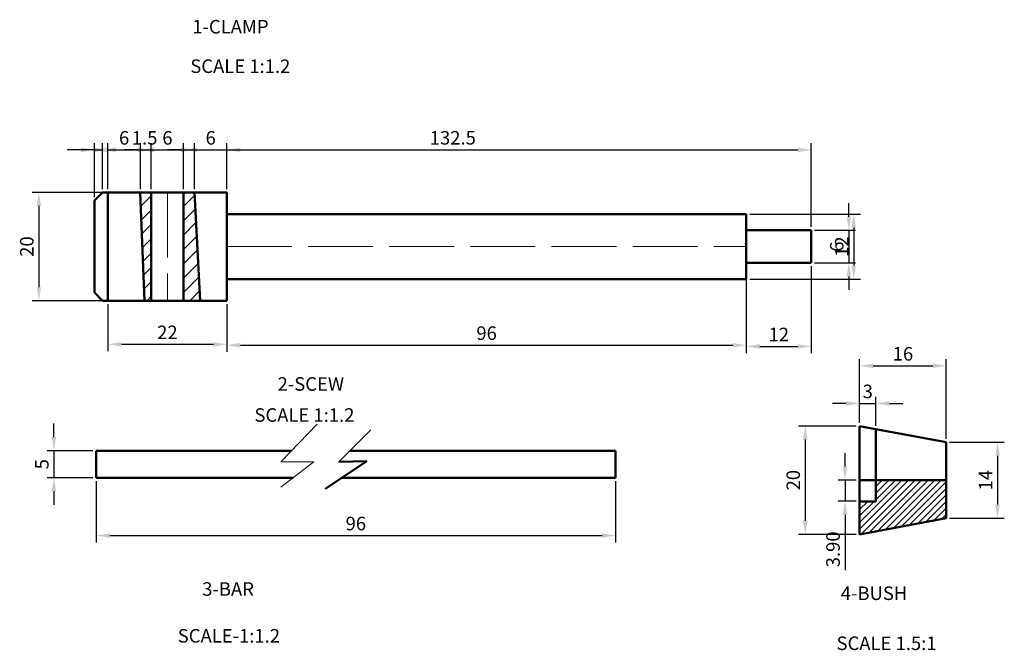
# Model space of a CAD drawing. Units: millimetres. Extents: x 1139 to 1488, y 1435 to 1756.
# Tile 1 of 3: x 1152 to 1334, y 1489 to 1606. Entities that reach past the tile are written whole.
import ezdxf

# ---------------------------------------------------------------- set-up
doc = ezdxf.new("R2010")
doc.units = ezdxf.units.MM
doc.linetypes.add('ACAD_ISO02W100', pattern=[15, 12, -3])
for name, color, linetype, lineweight in [('M-BREAK', 8, 'ACAD_ISO02W100', 18), ('M-CNTR', 4, 'ACAD_ISO02W100', 18), ('M-DIMS', 2, 'Continuous', 25), ('M-HATC', 8, 'Continuous', 18), ('M-OUTL', 7, 'Continuous', 50), ('M-TEXT', 7, 'Continuous', 25)]:
    doc.layers.add(name, color=color, linetype=linetype, lineweight=lineweight)
doc.styles.get("Standard").update_dxf_attribs({"font": 'arial.ttf'})
doc.dimstyles.new('ISO-25', dxfattribs={"dimtxt": 2.5, "dimasz": 2.5, "dimexe": 1.25, "dimexo": 0.625, "dimtad": 1, "dimtxsty": 'Standard', "dimcen": 2.5, "dimadec": 0, "dimazin": 0, "dimtfac": 1, "dimtmove": 0, "dimatfit": 3, "dimfxl": 1, "dimarcsym": 0})

# ---------------------------------------------------------------- blocks, each defined once
blk = doc.blocks.new('*D11')
at = {"layer": 'Defpoints', "color": 0, "transparency": 16777216}
for p in [(1168, 1554), (1190, 1554), (1190, 1545.95)]:
    blk.add_point(p, dxfattribs=at)
at = {"layer": 'M-DIMS', "color": 0, "lineweight": -2, "transparency": 16777216}
for p, q in [((1168, 1553.38), (1168, 1544.7)), ((1190, 1553.38), (1190, 1544.7)), ((1170.5, 1545.95), (1187.5, 1545.95))]:
    blk.add_line(p, q, dxfattribs=at)
at = {"layer": 'M-DIMS', "color": 0, "transparency": 16777216}
for points in [[(1170.5, 1546.37), (1170.5, 1545.53), (1168, 1545.95)], [(1187.5, 1546.37), (1187.5, 1545.53), (1190, 1545.95)]]:
    blk.add_solid(points, dxfattribs=at)
at = {"layer": 'M-DIMS', "color": 0, "transparency": 16777216, "insert": (1179, 1547.83), "char_height": 2.5, "attachment_point": 5}
blk.add_mtext('22', dxfattribs=at)
blk = doc.blocks.new('*D12')
at = {"layer": 'Defpoints', "color": 0, "transparency": 16777216}
for p in [(1168, 1574), (1155.24, 1554), (1168, 1554)]:
    blk.add_point(p, dxfattribs=at)
at = {"layer": 'M-DIMS', "color": 0, "lineweight": -2, "transparency": 16777216}
for p, q in [((1167.37, 1574), (1153.99, 1574)), ((1155.24, 1571.5), (1155.24, 1556.5)), ((1167.37, 1554), (1153.99, 1554))]:
    blk.add_line(p, q, dxfattribs=at)
at = {"layer": 'M-DIMS', "color": 0, "transparency": 16777216}
for points in [[(1154.82, 1571.5), (1155.66, 1571.5), (1155.24, 1574)], [(1154.82, 1556.5), (1155.66, 1556.5), (1155.24, 1554)]]:
    blk.add_solid(points, dxfattribs=at)
at = {"layer": 'M-DIMS', "color": 0, "transparency": 16777216, "insert": (1153.34, 1564), "char_height": 2.5, "attachment_point": 5, "rotation": 90}
blk.add_mtext('20', dxfattribs=at)
blk = doc.blocks.new('*D13')
at = {"layer": 'Defpoints', "color": 0, "transparency": 16777216}
for p in [(1286, 1558), (1190, 1554), (1286, 1545.79)]:
    blk.add_point(p, dxfattribs=at)
at = {"layer": 'M-DIMS', "color": 0, "lineweight": -2, "transparency": 16777216}
for p, q in [((1286, 1557.38), (1286, 1544.54)), ((1190, 1553.38), (1190, 1544.54)), ((1192.5, 1545.79), (1283.5, 1545.79))]:
    blk.add_line(p, q, dxfattribs=at)
at = {"layer": 'M-DIMS', "color": 0, "transparency": 16777216}
for points in [[(1192.5, 1546.2), (1192.5, 1545.37), (1190, 1545.79)], [(1283.5, 1546.2), (1283.5, 1545.37), (1286, 1545.79)]]:
    blk.add_solid(points, dxfattribs=at)
at = {"layer": 'M-DIMS', "color": 0, "transparency": 16777216, "insert": (1238, 1547.69), "char_height": 2.5, "attachment_point": 5}
blk.add_mtext('96', dxfattribs=at)
blk = doc.blocks.new('*D14')
at = {"layer": 'Defpoints', "color": 0, "transparency": 16777216}
for p in [(1286, 1561), (1298, 1561), (1298, 1545.56)]:
    blk.add_point(p, dxfattribs=at)
at = {"layer": 'M-DIMS', "color": 0, "lineweight": -2, "transparency": 16777216}
for p, q in [((1286, 1560.38), (1286, 1544.31)), ((1298, 1560.38), (1298, 1544.31)), ((1288.5, 1545.56), (1295.5, 1545.56))]:
    blk.add_line(p, q, dxfattribs=at)
at = {"layer": 'M-DIMS', "color": 0, "transparency": 16777216}
for points in [[(1288.5, 1545.98), (1288.5, 1545.15), (1286, 1545.56)], [(1295.5, 1545.98), (1295.5, 1545.15), (1298, 1545.56)]]:
    blk.add_solid(points, dxfattribs=at)
at = {"layer": 'M-DIMS', "color": 0, "transparency": 16777216, "insert": (1292, 1547.44), "char_height": 2.5, "attachment_point": 5}
blk.add_mtext('12', dxfattribs=at)
blk = doc.blocks.new('*D15')
at = {"layer": 'Defpoints', "color": 0, "transparency": 16777216}
for p in [(1298, 1567), (1298, 1561), (1304.95, 1561)]:
    blk.add_point(p, dxfattribs=at)
at = {"layer": 'M-DIMS', "color": 0, "lineweight": -2, "transparency": 16777216}
for p, q in [((1304.95, 1569.5), (1304.95, 1572)), ((1298.62, 1567), (1306.2, 1567)), ((1304.95, 1567), (1304.95, 1561)), ((1298.62, 1561), (1306.2, 1561)), ((1304.95, 1558.5), (1304.95, 1556))]:
    blk.add_line(p, q, dxfattribs=at)
at = {"layer": 'M-DIMS', "color": 0, "transparency": 16777216}
for points in [[(1304.54, 1569.5), (1305.37, 1569.5), (1304.95, 1567)], [(1304.54, 1558.5), (1305.37, 1558.5), (1304.95, 1561)]]:
    blk.add_solid(points, dxfattribs=at)
at = {"layer": 'M-DIMS', "color": 0, "transparency": 16777216, "insert": (1303.05, 1564), "char_height": 2.5, "attachment_point": 5, "rotation": 90}
blk.add_mtext('6', dxfattribs=at)
blk = doc.blocks.new('*D16')
at = {"layer": 'Defpoints', "color": 0, "transparency": 16777216}
for p in [(1165.83, 1521.31), (1261.83, 1521.31), (1261.83, 1510.63)]:
    blk.add_point(p, dxfattribs=at)
at = {"layer": 'M-DIMS', "color": 0, "lineweight": -2, "transparency": 16777216}
for p, q in [((1165.83, 1520.68), (1165.83, 1509.38)), ((1261.83, 1520.68), (1261.83, 1509.38)), ((1168.33, 1510.63), (1259.33, 1510.63))]:
    blk.add_line(p, q, dxfattribs=at)
at = {"layer": 'M-DIMS', "color": 0, "transparency": 16777216}
for points in [[(1168.33, 1511.05), (1168.33, 1510.21), (1165.83, 1510.63)], [(1259.33, 1511.05), (1259.33, 1510.21), (1261.83, 1510.63)]]:
    blk.add_solid(points, dxfattribs=at)
at = {"layer": 'M-DIMS', "color": 0, "transparency": 16777216, "insert": (1213.83, 1512.53), "char_height": 2.5, "attachment_point": 5}
blk.add_mtext('96', dxfattribs=at)
blk = doc.blocks.new('*D17')
at = {"layer": 'Defpoints', "color": 0, "transparency": 16777216}
for p in [(1165.83, 1526.31), (1158.02, 1521.31), (1165.83, 1521.31)]:
    blk.add_point(p, dxfattribs=at)
at = {"layer": 'M-DIMS', "color": 0, "lineweight": -2, "transparency": 16777216}
for p, q in [((1158.02, 1528.81), (1158.02, 1531.31)), ((1165.21, 1526.31), (1156.77, 1526.31)), ((1158.02, 1526.31), (1158.02, 1521.31)), ((1165.21, 1521.31), (1156.77, 1521.31)), ((1158.02, 1518.81), (1158.02, 1516.31))]:
    blk.add_line(p, q, dxfattribs=at)
at = {"layer": 'M-DIMS', "color": 0, "transparency": 16777216}
for points in [[(1157.6, 1528.81), (1158.44, 1528.81), (1158.02, 1526.31)], [(1157.6, 1518.81), (1158.44, 1518.81), (1158.02, 1521.31)]]:
    blk.add_solid(points, dxfattribs=at)
at = {"layer": 'M-DIMS', "color": 0, "transparency": 16777216, "insert": (1156.12, 1523.81), "char_height": 2.5, "attachment_point": 5, "rotation": 90}
blk.add_mtext('5', dxfattribs=at)
blk = doc.blocks.new('*D18')
at = {"layer": 'Defpoints', "color": 0, "transparency": 16777216}
for p in [(1306.95, 1530.86), (1296.9, 1510.86), (1306.95, 1510.86)]:
    blk.add_point(p, dxfattribs=at)
at = {"layer": 'M-DIMS', "color": 0, "lineweight": -2, "transparency": 16777216}
for p, q in [((1306.32, 1530.86), (1295.65, 1530.86)), ((1296.9, 1528.36), (1296.9, 1513.36)), ((1306.32, 1510.86), (1295.65, 1510.86))]:
    blk.add_line(p, q, dxfattribs=at)
at = {"layer": 'M-DIMS', "color": 0, "transparency": 16777216}
for points in [[(1296.48, 1528.36), (1297.32, 1528.36), (1296.9, 1530.86)], [(1296.48, 1513.36), (1297.32, 1513.36), (1296.9, 1510.86)]]:
    blk.add_solid(points, dxfattribs=at)
at = {"layer": 'M-DIMS', "color": 0, "transparency": 16777216, "insert": (1295, 1520.86), "char_height": 2.5, "attachment_point": 5, "rotation": 90}
blk.add_mtext('20', dxfattribs=at)
blk = doc.blocks.new('*D19')
at = {"layer": 'Defpoints', "color": 0, "transparency": 16777216}
for p in [(1309.95, 1535.03), (1306.95, 1530.86), (1309.95, 1530.29)]:
    blk.add_point(p, dxfattribs=at)
at = {"layer": 'M-DIMS', "color": 0, "lineweight": -2, "transparency": 16777216}
for p, q in [((1306.95, 1531.48), (1306.95, 1536.28)), ((1309.95, 1530.92), (1309.95, 1536.28)), ((1304.45, 1535.03), (1301.95, 1535.03)), ((1306.95, 1535.03), (1309.95, 1535.03)), ((1312.45, 1535.03), (1314.95, 1535.03))]:
    blk.add_line(p, q, dxfattribs=at)
at = {"layer": 'M-DIMS', "color": 0, "transparency": 16777216}
for points in [[(1304.45, 1535.45), (1304.45, 1534.61), (1306.95, 1535.03)], [(1312.45, 1535.45), (1312.45, 1534.61), (1309.95, 1535.03)]]:
    blk.add_solid(points, dxfattribs=at)
at = {"layer": 'M-DIMS', "color": 0, "transparency": 16777216, "insert": (1308.45, 1536.93), "char_height": 2.5, "attachment_point": 5}
blk.add_mtext('3', dxfattribs=at)
blk = doc.blocks.new('*D20')
at = {"layer": 'Defpoints', "color": 0, "transparency": 16777216}
for p in [(1322.95, 1527.86), (1322.95, 1513.86), (1332.43, 1513.86)]:
    blk.add_point(p, dxfattribs=at)
at = {"layer": 'M-DIMS', "color": 0, "lineweight": -2, "transparency": 16777216}
for p, q in [((1323.57, 1527.86), (1333.68, 1527.86)), ((1332.43, 1525.36), (1332.43, 1516.36)), ((1323.57, 1513.86), (1333.68, 1513.86))]:
    blk.add_line(p, q, dxfattribs=at)
at = {"layer": 'M-DIMS', "color": 0, "transparency": 16777216}
for points in [[(1332.02, 1525.36), (1332.85, 1525.36), (1332.43, 1527.86)], [(1332.02, 1516.36), (1332.85, 1516.36), (1332.43, 1513.86)]]:
    blk.add_solid(points, dxfattribs=at)
at = {"layer": 'M-DIMS', "color": 0, "transparency": 16777216, "insert": (1330.55, 1520.86), "char_height": 2.5, "attachment_point": 5, "rotation": 90}
blk.add_mtext('14', dxfattribs=at)
blk = doc.blocks.new('*D21')
at = {"layer": 'Defpoints', "color": 0, "transparency": 16777216}
for p in [(1322.95, 1541.98), (1306.95, 1530.86), (1322.95, 1527.86)]:
    blk.add_point(p, dxfattribs=at)
at = {"layer": 'M-DIMS', "color": 0, "lineweight": -2, "transparency": 16777216}
for p, q in [((1306.95, 1531.48), (1306.95, 1543.23)), ((1309.45, 1541.98), (1320.45, 1541.98)), ((1322.95, 1528.48), (1322.95, 1543.23))]:
    blk.add_line(p, q, dxfattribs=at)
at = {"layer": 'M-DIMS', "color": 0, "transparency": 16777216}
for points in [[(1309.45, 1542.4), (1309.45, 1541.56), (1306.95, 1541.98)], [(1320.45, 1542.4), (1320.45, 1541.56), (1322.95, 1541.98)]]:
    blk.add_solid(points, dxfattribs=at)
at = {"layer": 'M-DIMS', "color": 0, "transparency": 16777216, "insert": (1314.95, 1543.88), "char_height": 2.5, "attachment_point": 5}
blk.add_mtext('16', dxfattribs=at)
blk = doc.blocks.new('*D40')
at = {"layer": 'Defpoints', "color": 0, "transparency": 16777216}
for p in [(1298, 1581.85), (1165.5, 1572.5), (1298, 1567)]:
    blk.add_point(p, dxfattribs=at)
at = {"layer": 'M-DIMS', "color": 0, "lineweight": -2, "transparency": 16777216}
for p, q in [((1165.5, 1573.13), (1165.5, 1583.1)), ((1168, 1581.85), (1295.5, 1581.85)), ((1298, 1567.63), (1298, 1583.1))]:
    blk.add_line(p, q, dxfattribs=at)
at = {"layer": 'M-DIMS', "color": 0, "transparency": 16777216}
for points in [[(1168, 1582.27), (1168, 1581.44), (1165.5, 1581.85)], [(1295.5, 1582.27), (1295.5, 1581.44), (1298, 1581.85)]]:
    blk.add_solid(points, dxfattribs=at)
at = {"layer": 'M-DIMS', "color": 0, "transparency": 16777216, "insert": (1231.75, 1583.76), "char_height": 2.5, "attachment_point": 5}
blk.add_mtext('132.5', dxfattribs=at)
blk = doc.blocks.new('*D41')
at = {"layer": 'Defpoints', "color": 0, "transparency": 16777216}
for p in [(1167, 1581.85), (1165.5, 1572.5), (1167, 1574)]:
    blk.add_point(p, dxfattribs=at)
at = {"layer": 'M-DIMS', "color": 0, "lineweight": -2, "transparency": 16777216}
for p, q in [((1163, 1581.85), (1160.5, 1581.85)), ((1165.5, 1573.13), (1165.5, 1583.1)), ((1165.5, 1581.85), (1167, 1581.85)), ((1167, 1574.63), (1167, 1583.1)), ((1169.5, 1581.85), (1177.58, 1581.85))]:
    blk.add_line(p, q, dxfattribs=at)
at = {"layer": 'M-DIMS', "color": 0, "transparency": 16777216}
for points in [[(1163, 1582.27), (1163, 1581.44), (1165.5, 1581.85)], [(1169.5, 1582.27), (1169.5, 1581.44), (1167, 1581.85)]]:
    blk.add_solid(points, dxfattribs=at)
at = {"layer": 'M-DIMS', "color": 0, "transparency": 16777216, "insert": (1174.79, 1583.75), "char_height": 2.5, "attachment_point": 5}
blk.add_mtext('1.5', dxfattribs=at)
blk = doc.blocks.new('*D42')
at = {"layer": 'Defpoints', "color": 0, "transparency": 16777216}
for p in [(1174, 1581.85), (1168, 1574), (1174, 1574)]:
    blk.add_point(p, dxfattribs=at)
at = {"layer": 'M-DIMS', "color": 0, "lineweight": -2, "transparency": 16777216}
for p, q in [((1165.5, 1581.85), (1163, 1581.85)), ((1168, 1574.63), (1168, 1583.1)), ((1168, 1581.85), (1174, 1581.85)), ((1174, 1574.63), (1174, 1583.1)), ((1176.5, 1581.85), (1179, 1581.85))]:
    blk.add_line(p, q, dxfattribs=at)
at = {"layer": 'M-DIMS', "color": 0, "transparency": 16777216}
for points in [[(1165.5, 1582.27), (1165.5, 1581.44), (1168, 1581.85)], [(1176.5, 1582.27), (1176.5, 1581.44), (1174, 1581.85)]]:
    blk.add_solid(points, dxfattribs=at)
at = {"layer": 'M-DIMS', "color": 0, "transparency": 16777216, "insert": (1171, 1583.75), "char_height": 2.5, "attachment_point": 5}
blk.add_mtext('6', dxfattribs=at)
blk = doc.blocks.new('*D43')
at = {"layer": 'Defpoints', "color": 0, "transparency": 16777216}
for p in [(1182, 1581.85), (1176, 1574), (1182, 1574)]:
    blk.add_point(p, dxfattribs=at)
at = {"layer": 'M-DIMS', "color": 0, "lineweight": -2, "transparency": 16777216}
for p, q in [((1173.5, 1581.85), (1171, 1581.85)), ((1176, 1574.63), (1176, 1583.1)), ((1176, 1581.85), (1182, 1581.85)), ((1182, 1574.63), (1182, 1583.1)), ((1184.5, 1581.85), (1187, 1581.85))]:
    blk.add_line(p, q, dxfattribs=at)
at = {"layer": 'M-DIMS', "color": 0, "transparency": 16777216}
for points in [[(1173.5, 1582.27), (1173.5, 1581.44), (1176, 1581.85)], [(1184.5, 1582.27), (1184.5, 1581.44), (1182, 1581.85)]]:
    blk.add_solid(points, dxfattribs=at)
at = {"layer": 'M-DIMS', "color": 0, "transparency": 16777216, "insert": (1179, 1583.75), "char_height": 2.5, "attachment_point": 5}
blk.add_mtext('6', dxfattribs=at)
blk = doc.blocks.new('*D44')
at = {"layer": 'Defpoints', "color": 0, "transparency": 16777216}
for p in [(1190, 1581.85), (1184, 1574), (1190, 1574)]:
    blk.add_point(p, dxfattribs=at)
at = {"layer": 'M-DIMS', "color": 0, "lineweight": -2, "transparency": 16777216}
for p, q in [((1181.5, 1581.85), (1179, 1581.85)), ((1184, 1574.63), (1184, 1583.1)), ((1184, 1581.85), (1190, 1581.85)), ((1190, 1574.63), (1190, 1583.1)), ((1192.5, 1581.85), (1195, 1581.85))]:
    blk.add_line(p, q, dxfattribs=at)
at = {"layer": 'M-DIMS', "color": 0, "transparency": 16777216}
for points in [[(1181.5, 1582.27), (1181.5, 1581.44), (1184, 1581.85)], [(1192.5, 1582.27), (1192.5, 1581.44), (1190, 1581.85)]]:
    blk.add_solid(points, dxfattribs=at)
at = {"layer": 'M-DIMS', "color": 0, "transparency": 16777216, "insert": (1187, 1583.75), "char_height": 2.5, "attachment_point": 5}
blk.add_mtext('6', dxfattribs=at)
blk = doc.blocks.new('*D45')
at = {"layer": 'Defpoints', "color": 0, "transparency": 16777216}
for p in [(1286, 1570), (1286, 1558), (1305.85, 1558)]:
    blk.add_point(p, dxfattribs=at)
at = {"layer": 'M-DIMS', "color": 0, "lineweight": -2, "transparency": 16777216}
for p, q in [((1286.62, 1570), (1307.1, 1570)), ((1305.85, 1567.5), (1305.85, 1560.5)), ((1286.62, 1558), (1307.1, 1558))]:
    blk.add_line(p, q, dxfattribs=at)
at = {"layer": 'M-DIMS', "color": 0, "transparency": 16777216}
for points in [[(1305.43, 1567.5), (1306.26, 1567.5), (1305.85, 1570)], [(1305.43, 1560.5), (1306.26, 1560.5), (1305.85, 1558)]]:
    blk.add_solid(points, dxfattribs=at)
at = {"layer": 'M-DIMS', "color": 0, "transparency": 16777216, "insert": (1303.97, 1564), "char_height": 2.5, "attachment_point": 5, "rotation": 90}
blk.add_mtext('12', dxfattribs=at)
blk = doc.blocks.new('*D46')
at = {"layer": 'Defpoints', "color": 0, "transparency": 16777216}
for p in [(1306.95, 1520.86), (1304.25, 1516.96), (1306.95, 1516.96)]:
    blk.add_point(p, dxfattribs=at)
at = {"layer": 'M-DIMS', "color": 0, "lineweight": -2, "transparency": 16777216}
for p, q in [((1304.25, 1523.36), (1304.25, 1525.86)), ((1306.32, 1520.86), (1303, 1520.86)), ((1304.25, 1520.86), (1304.25, 1516.96)), ((1306.32, 1516.96), (1303, 1516.96)), ((1304.25, 1514.46), (1304.25, 1504.22))]:
    blk.add_line(p, q, dxfattribs=at)
at = {"layer": 'M-DIMS', "color": 0, "transparency": 16777216}
for points in [[(1303.83, 1523.36), (1304.66, 1523.36), (1304.25, 1520.86)], [(1303.83, 1514.46), (1304.66, 1514.46), (1304.25, 1516.96)]]:
    blk.add_solid(points, dxfattribs=at)
at = {"layer": 'M-DIMS', "color": 0, "transparency": 16777216, "insert": (1302.35, 1508.09), "char_height": 2.5, "attachment_point": 5, "rotation": 90}
blk.add_mtext('3.90', dxfattribs=at)

msp = doc.modelspace()

# ---------------------------------------------------------------- hatches: boundary and pattern name
at = {"layer": 'M-HATC'}
h = msp.add_hatch(dxfattribs=at)
h.set_pattern_fill('ANSI31', color=256, scale=0.59)
h.paths.add_polyline_path([(1175.9953, 1574.0031), (1173.9953, 1574.0031), (1174.7527, 1554.0031), (1175.9953, 1554.0031)])
h = msp.add_hatch(dxfattribs=at)
h.set_pattern_fill('ANSI31', color=256, scale=0.59)
h.paths.add_polyline_path([(1183.9953, 1574.0031), (1181.9953, 1574.0031), (1181.9953, 1554.0031), (1185.0338, 1554.0031)])
h = msp.add_hatch(dxfattribs=at)
h.set_pattern_fill('ANSI31', color=256, scale=0.27)
h.paths.add_polyline_path([(1322.9481, 1520.8552), (1309.9481, 1520.8552), (1309.9481, 1516.9557), (1306.9481, 1516.9557), (1306.9481, 1510.8552), (1322.9481, 1513.8552)])

# ---------------------------------------------------------------- linework, layer by layer
at = {"layer": 'M-BREAK'}
for p, q in [((1206.7017, 1531.2097), (1199.9403, 1524.2463)), ((1216.5837, 1530.1704), (1210.6545, 1524.2463)), ((1199.9403, 1524.2463), (1206.0775, 1524.2463)), ((1206.0775, 1524.2463), (1199.9403, 1519.5695))]:
    msp.add_line(p, q, dxfattribs=at)
at = {"layer": 'M-CNTR'}
for p, q in [((1178.9953, 1574.0031), (1178.9953, 1554.0031)), ((1189.9953, 1564.0031), (1285.9953, 1564.0031))]:
    msp.add_line(p, q, dxfattribs=at)
at = {"layer": 'M-OUTL'}
for p, q in [((1166.9953, 1574.0031), (1165.4953, 1572.5031)), ((1165.4953, 1572.5031), (1165.4953, 1555.5031)), ((1167.9953, 1574.0031), (1166.9953, 1574.0031)), ((1167.9953, 1574.0031), (1189.9953, 1574.0031)), ((1167.9953, 1554.0031), (1167.9953, 1574.0031)), ((1175.9953, 1574.0031), (1173.9953, 1574.0031)), ((1173.9953, 1574.0031), (1174.7527, 1554.0031)), ((1178.9953, 1574.0031), (1175.9953, 1574.0031)), ((1175.9953, 1574.0031), (1175.9953, 1554.0031)), ((1181.9953, 1554.0031), (1181.9953, 1574.0031)), ((1181.9953, 1574.0031), (1183.9953, 1574.0031)), ((1183.9953, 1574.0031), (1185.0338, 1554.0031)), ((1189.9953, 1574.0031), (1189.9953, 1554.0031)), ((1285.9953, 1570.0031), (1189.9953, 1570.0031)), ((1285.9953, 1564.0031), (1285.9953, 1570.0031)), ((1285.9953, 1564.0031), (1285.9953, 1567.0031)), ((1285.9953, 1567.0031), (1297.9953, 1567.0031)), ((1297.9953, 1567.0031), (1297.9953, 1561.0031)), ((1285.9953, 1564.0031), (1285.9953, 1558.0031)), ((1297.9953, 1561.0031), (1285.9953, 1561.0031)), ((1285.9953, 1558.0031), (1189.9953, 1558.0031)), ((1166.9953, 1554.0031), (1165.4953, 1555.5031)), ((1166.9953, 1554.0031), (1167.9953, 1554.0031)), ((1189.9953, 1554.0031), (1167.9953, 1554.0031)), ((1306.9481, 1530.8552), (1306.9481, 1510.8552)), ((1306.9481, 1530.8552), (1322.9481, 1527.8552)), ((1309.9481, 1530.2927), (1309.9481, 1516.9557)), ((1322.9481, 1520.8552), (1322.9481, 1527.8552)), ((1165.8318, 1526.306), (1201.9402, 1526.306)), ((1165.8318, 1521.306), (1165.8318, 1526.306)), ((1212.7159, 1526.306), (1261.8318, 1526.306)), ((1261.8318, 1526.306), (1261.8318, 1521.306)), ((1215.8555, 1524.3503), (1208.158, 1519.2577)), ((1210.6545, 1524.2463), (1215.8555, 1524.3503)), ((1202.219, 1521.306), (1165.8318, 1521.306)), ((1261.8318, 1521.306), (1211.254, 1521.306)), ((1306.9481, 1520.8552), (1322.9481, 1520.8552)), ((1322.9481, 1520.8552), (1322.9481, 1513.8552)), ((1309.9481, 1516.9557), (1306.9481, 1516.9557)), ((1322.9481, 1513.8552), (1306.9481, 1510.8552))]:
    msp.add_line(p, q, dxfattribs=at)

# ---------------------------------------------------------------- texts
at = {"layer": 'M-TEXT', "char_height": 2.5, "attachment_point": 1}
for s, width, insert in [('1-CLAMP', 102.092946, (1183.599, 1605.8474)), ('SCALE 1:1.2', 25.704473, (1183.2335, 1598.5588)), ('2-SCEW', 39.565091, (1199.3619, 1539.8789)), ('SCALE 1:1.2', 31.993992, (1195.0879, 1534.1446)), ('3-BAR', 44.850297, (1185.4359, 1502.018)), ('4-BUSH', 30.0969, (1303.463, 1501.2319)), ('SCALE-1:1.2', 44.653583, (1180.9115, 1493.3703)), ('SCALE 1.5:1', 23.605421, (1302.6761, 1491.9945))]:
    msp.add_mtext_dynamic_manual_height_columns(s, width=width, gutter_width=12.5, heights=[0], dxfattribs=dict(at, insert=insert))

# ---------------------------------------------------------------- dimensions: what is measured, and where the dimension line sits
at = {"layer": 'M-DIMS'}
for base, p1, p2, override, picture, middle in [((1166.9953, 1581.8531), (1165.4953, 1572.5031), (1166.9953, 1574.0031), {"dimdec": 1, "dimlfac": 1, "dimrnd": 0, "dimzin": 0, "dimdsep": 46, "dimlunit": 2}, '*D41', (1174.7877, 1583.7545)), ((1173.9953, 1581.8531), (1167.9953, 1574.0031), (1173.9953, 1574.0031), {"dimdec": 0, "dimlfac": 1, "dimrnd": 0, "dimzin": 0, "dimdsep": 46, "dimlunit": 2}, '*D42', (1170.9953, 1583.7545)), ((1297.9953, 1581.8531), (1165.4953, 1572.5031), (1297.9953, 1567.0031), {"dimdec": 1, "dimlfac": 1, "dimrnd": 0, "dimzin": 0, "dimdsep": 46, "dimlunit": 2}, '*D40', (1231.7453, 1583.7553)), ((1181.9953, 1581.8531), (1175.9953, 1574.0031), (1181.9953, 1574.0031), {"dimdec": 0, "dimlfac": 1, "dimrnd": 0, "dimzin": 0, "dimdsep": 46, "dimlunit": 2}, '*D43', (1178.9953, 1583.7545)), ((1189.9953, 1581.8531), (1183.9953, 1574.0031), (1189.9953, 1574.0031), {"dimdec": 0, "dimlfac": 1, "dimrnd": 0, "dimzin": 0, "dimdsep": 46, "dimlunit": 2}, '*D44', (1186.9953, 1583.7545)), ((1297.9953, 1545.5627), (1285.9953, 1561.0031), (1297.9953, 1561.0031), {"dimclrd": 0, "dimclre": 0, "dimclrt": 0}, '*D14', (1291.9953, 1547.4428)), ((1285.9953, 1545.7869), (1189.9953, 1554.0031), (1285.9953, 1558.0031), {"dimclrd": 0, "dimclre": 0, "dimclrt": 0}, '*D13', (1237.9953, 1547.6884)), ((1189.9953, 1545.951), (1167.9953, 1554.0031), (1189.9953, 1554.0031), {"dimclrd": 0, "dimclre": 0, "dimclrt": 0}, '*D11', (1178.9953, 1547.8312)), ((1322.9481, 1541.9792), (1306.9481, 1530.8552), (1322.9481, 1527.8552), {"dimclrd": 0, "dimclre": 0, "dimclrt": 0}, '*D21', (1314.9481, 1543.8807)), ((1309.9481, 1535.0284), (1306.9481, 1530.8552), (1309.9481, 1530.2927), {"dimclrd": 0, "dimclre": 0, "dimclrt": 0}, '*D19', (1308.4481, 1536.9307)), ((1261.8318, 1510.6315), (1165.8318, 1521.306), (1261.8318, 1521.306), {"dimclrd": 0, "dimclre": 0, "dimclrt": 0}, '*D16', (1213.8318, 1512.5329))]:
    dim = msp.add_linear_dim(base=base, p1=p1, p2=p2, dimstyle='ISO-25', override=override, dxfattribs=at)
    dim.commit()
    dim.dimension.update_dxf_attribs({"geometry": picture, "text_midpoint": middle})
for base, p1, p2, override, picture, middle in [((1155.2405, 1554.0031), (1167.9953, 1574.0031), (1167.9953, 1554.0031), {"dimclrd": 0, "dimclre": 0, "dimclrt": 0}, '*D12', (1153.3391, 1564.0031)), ((1304.9535, 1561.0031), (1297.9953, 1567.0031), (1297.9953, 1561.0031), {"dimclrd": 0, "dimclre": 0, "dimclrt": 0}, '*D15', (1303.0521, 1564.0031)), ((1305.8453, 1558.0031), (1285.9953, 1570.0031), (1285.9953, 1558.0031), {"dimdec": 0, "dimlfac": 1, "dimrnd": 0, "dimzin": 0, "dimdsep": 46, "dimlunit": 2}, '*D45', (1303.9651, 1564.0031)), ((1158.0198, 1521.306), (1165.8318, 1526.306), (1165.8318, 1521.306), {"dimclrd": 0, "dimclre": 0, "dimclrt": 0}, '*D17', (1156.1235, 1523.806)), ((1296.9008, 1510.8552), (1306.9481, 1530.8552), (1306.9481, 1510.8552), {"dimclrd": 0, "dimclre": 0, "dimclrt": 0}, '*D18', (1294.9994, 1520.8552)), ((1332.4346, 1513.8552), (1322.9481, 1527.8552), (1322.9481, 1513.8552), {"dimclrd": 0, "dimclre": 0, "dimclrt": 0}, '*D20', (1330.5544, 1520.8552)), ((1304.2481, 1516.9557), (1306.9481, 1520.8552), (1306.9481, 1516.9557), {"dimdec": 2, "dimlfac": 1, "dimrnd": 0, "dimzin": 0, "dimdsep": 46, "dimlunit": 2}, '*D46', (1302.3458, 1508.0889))]:
    dim = msp.add_linear_dim(base=base, p1=p1, p2=p2, angle=90, dimstyle='ISO-25', override=override, dxfattribs=at)
    dim.commit()
    dim.dimension.update_dxf_attribs({"geometry": picture, "text_midpoint": middle})

doc.saveas('drawing.dxf')
